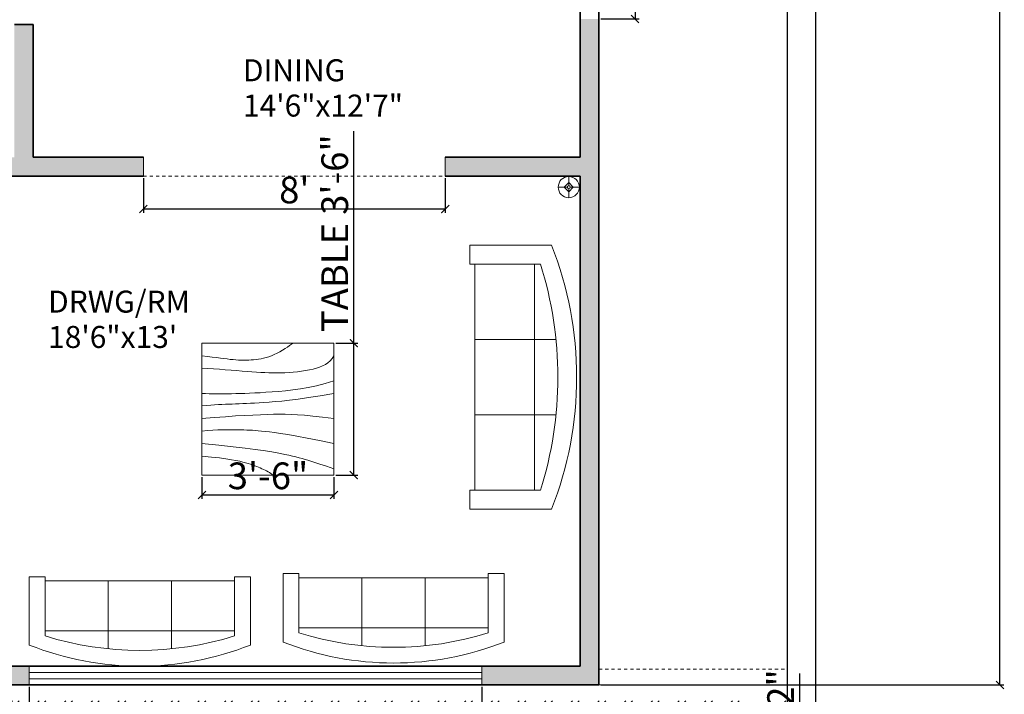
# Model space of a CAD drawing. Units: inches. Extents: x 3799 to 20199, y 1682 to 8087.
# Tile 9 of 30: x 11366 to 11679, y 2322 to 2537. Entities that reach past the tile are written whole.
import ezdxf

# ---------------------------------------------------------------- set-up
doc = ezdxf.new("R2010")
doc.units = ezdxf.units.IN
doc.linetypes.add('JIS_02_1.0', pattern=[2, 1, -1])
for name, color, linetype, lineweight in [('A-ANNO-DIMS', 2, 'Continuous', 18), ('A-AREA-IDEN', 7, 'Continuous', 18), ('A-DOOR', 3, 'Continuous', 18), ('A-FURN', 8, 'Continuous', 18), ('A-GLAZ', 152, 'Continuous', 18), ('A-SITE-OVHD', 8, 'JIS_02_1.0', 18), ('A-WALL', 7, 'Continuous', 35), ('A-WALL-OVHD', 7, 'JIS_02_1.0', 18), ('A-WALL-PATT', 252, 'Continuous', 13), ('C-PROP', 7, 'Continuous', 25), ('L-PLNT-PATT', 94, 'Continuous', 13)]:
    doc.layers.add(name, color=color, linetype=linetype, lineweight=lineweight)
doc.styles.get("Standard").update_dxf_attribs({"font": 'arial.ttf'})
doc.dimstyles.new('ISO-25', dxfattribs={"dimtxt": 8.5, "dimasz": 2.5, "dimexe": 1.25, "dimexo": 0.625, "dimtad": 1, "dimdec": 0, "dimlunit": 3, "dimtxsty": 'Standard', "dimblk": 'ARCHTICK', "dimcen": 2.5, "dimadec": 0, "dimazin": 0, "dimtfac": 1, "dimtdec": 0, "dimtmove": 0, "dimatfit": 3, "dimfxl": 1, "dimarcsym": 0})

# ---------------------------------------------------------------- blocks, each defined once
blk = doc.blocks.new('Sofa - Roundback 7 ft.')
for p, q in [((-12.00002, -32.4421), (-12.00003, -6.5971)), ((11.99997, -32.4421), (11.99998, -6.5971)), ((-36.000027, -34), (-36.000027, -11.4696)), ((35.99998, -34), (35.99998, -11.4696)), ((-35.999844, -13.3819), (35.9998, -13.3819)), ((-36.000027, -32.4421), (35.99998, -32.4421))]:
    blk.add_line(p, q)
for points in [[(-36.000027, -34), (-42.000027, -34), (-42.000027, -8)], [(41.99998, -8), (41.99998, -34), (35.99998, -34)]]:
    blk.add_lwpolyline(points)
for centre, radius, start, end in [((0, -114.25), 114.25, 68.43141, 111.5686), ((-0.00001, -127.1968), 121.1968, 72.72033, 107.2797)]:
    blk.add_arc(centre, radius, start, end)
blk = doc.blocks.new('Table - Square Woodgrain 42 x 42 in.')
blk.add_line((0, -42), (42, -42))
for points in [[(0, -4), (1.704, -4.2172), (3.2358, -4.4188), (4.615, -4.604), (5.8615, -4.7721), (6.9951, -4.9224), (8.0357, -5.0541), (9.0031, -5.1667), (9.9171, -5.2594), (10.7951, -5.3316), (11.6445, -5.3836), (12.4702, -5.4157), (13.277, -5.4283), (14.0698, -5.4217), (14.8535, -5.3964), (15.6331, -5.3526), (16.4133, -5.2908), (17.1986, -5.2103), (17.9913, -5.1062), (18.793, -4.9727), (19.6056, -4.8038), (20.4307, -4.5937), (21.2701, -4.3365), (22.1256, -4.0262), (22.9989, -3.6571), (23.888, -3.2272), (24.7756, -2.7516), (25.6408, -2.2491), (26.4624, -1.7387), (27.2195, -1.2395), (27.891, -0.7703), (28.456, -0.3501), (28.8934, 0.002)], [(0, -42), (0, 0), (42, 0), (42, -42)], [(0, -8), (1.8203, -8.1001), (3.6741, -8.2149), (5.5411, -8.3408), (7.4011, -8.4741), (9.2339, -8.6112), (11.0193, -8.7484), (12.7371, -8.8821), (14.3671, -9.0086), (15.8954, -9.1246), (17.3337, -9.2278), (18.6997, -9.3159), (20.0116, -9.387), (21.2871, -9.4389), (22.5442, -9.4696), (23.8008, -9.477), (25.0749, -9.459), (26.3791, -9.4137), (27.7049, -9.3403), (29.0383, -9.2382), (30.3655, -9.1068), (31.6728, -8.9455), (32.9461, -8.7535), (34.1717, -8.5304), (35.3358, -8.2756), (36.4268, -7.9863), (37.443, -7.6521), (38.3849, -7.2603), (39.253, -6.7986), (40.048, -6.2542), (40.7705, -5.6147), (41.421, -4.8674), (42, -4)], [(42, -12), (39.1784, -12.8621), (36.4519, -13.5654), (33.8246, -14.1294), (31.3004, -14.5731), (28.8832, -14.9161), (26.577, -15.1775), (24.3858, -15.3768), (22.3136, -15.5332), (20.3622, -15.6632), (18.5254, -15.7718), (16.7947, -15.8612), (15.1618, -15.9338), (13.6183, -15.9916), (12.1558, -16.0369), (10.7659, -16.0718), (9.4403, -16.0987), (8.1703, -16.1191), (6.9461, -16.1325), (5.7577, -16.1377), (4.595, -16.1335), (3.4479, -16.1188), (2.3064, -16.0924), (1.1604, -16.0532), (0, -16)], [(42, -16), (37.6529, -16.7365), (33.8802, -17.329), (30.6179, -17.7961), (27.8015, -18.1561), (25.3668, -18.4275), (23.2497, -18.6288), (21.3859, -18.7785), (19.7111, -18.8949), (18.1693, -18.9939), (16.7375, -19.0795), (15.401, -19.1534), (14.1449, -19.217), (12.9544, -19.2717), (11.8148, -19.3191), (10.7113, -19.3606), (9.6291, -19.3976), (8.5534, -19.4323), (7.47, -19.4689), (6.3643, -19.5122), (5.222, -19.5672), (4.0288, -19.6386), (2.7703, -19.7313), (1.4321, -19.8501), (0, -20)], [(0, -24), (3.9243, -23.6805), (7.4766, -23.4138), (10.6891, -23.1954), (13.5943, -23.0205), (16.2247, -22.8847), (18.6125, -22.7832), (20.7903, -22.7116), (22.7903, -22.6651), (24.6563, -22.642), (26.4764, -22.6507), (28.35, -22.7024), (30.3766, -22.8084), (32.6555, -22.98), (35.2861, -23.2283), (38.3678, -23.5645), (42, -24)], [(42, -32), (37.392, -31.017), (33.4585, -30.2231), (30.1291, -29.5949), (27.3334, -29.109), (25.0009, -28.742), (23.0612, -28.4707), (21.4439, -28.2716), (20.0786, -28.1215), (18.8998, -28.0002), (17.8609, -27.9014), (16.9206, -27.8219), (16.0371, -27.7588), (15.1691, -27.709), (14.2748, -27.6693), (13.3128, -27.6368), (12.2415, -27.6083), (11.0295, -27.5824), (9.6867, -27.5643), (8.233, -27.5608), (6.6884, -27.5787), (5.0728, -27.6248), (3.4062, -27.7058), (1.7086, -27.8286), (0, -28)], [(0, -32), (5.4026, -32.5358), (9.9494, -33.019), (13.7424, -33.4553), (16.8834, -33.8505), (19.4743, -34.2106), (21.6171, -34.5413), (23.4136, -34.8486), (24.9657, -35.1382), (26.3614, -35.4156), (27.6332, -35.6841), (28.7995, -35.9467), (29.8788, -36.2064), (30.8897, -36.4661), (31.8507, -36.7288), (32.7802, -36.9973), (33.6968, -37.2747), (34.6175, -37.5635), (35.5531, -37.8651), (36.5128, -38.1805), (37.506, -38.5108), (38.5421, -38.8568), (39.6302, -39.2197), (40.7797, -39.6004), (42, -40)], [(0, -36), (3.0098, -36.2857), (5.5354, -36.5643), (7.6368, -36.8359), (9.374, -37.1009), (10.807, -37.3597), (11.9957, -37.6126), (13.0002, -37.8599), (13.8804, -38.102), (14.6874, -38.3393), (15.4365, -38.5729), (16.1338, -38.8041), (16.7858, -39.0341), (17.3987, -39.264), (17.9787, -39.4952), (18.5322, -39.7288), (19.0655, -39.9662), (19.5832, -40.2081), (20.0842, -40.4544), (20.5657, -40.7046), (21.0249, -40.9581), (21.459, -41.2144), (21.8653, -41.4731), (22.2409, -41.7335), (22.5831, -41.9951)]]:
    blk.add_lwpolyline(points)
blk = doc.blocks.new('_ArchTick')
at = {"color": 0, "linetype": 'ByBlock', "const_width": 0.15}
blk.add_lwpolyline([(-0.5, -0.5), (0.5, 0.5)], dxfattribs=at)
blk = doc.blocks.new('*D58')
at = {"layer": 'A-ANNO-DIMS', "color": 0, "lineweight": -2, "transparency": 16777216}
for p, q in [((11404.92, 2486.45), (11404.92, 2475.33)), ((11500.92, 2486.45), (11500.92, 2475.33)), ((11500.92, 2476.58), (11404.92, 2476.58))]:
    blk.add_line(p, q, dxfattribs=at)
at = {"layer": 'Defpoints', "color": 0, "transparency": 16777216}
for p in [(11404.92, 2487.07), (11500.92, 2487.07), (11404.92, 2476.58)]:
    blk.add_point(p, dxfattribs=at)
at = {"layer": 'A-ANNO-DIMS', "color": 0, "lineweight": -2, "transparency": 16777216, "xscale": 2.5, "yscale": 2.5, "zscale": 2.5, "rotation": 180}
blk.add_blockref('_ArchTick', (11404.92, 2476.58), dxfattribs=at)
at = {"layer": 'A-ANNO-DIMS', "color": 0, "lineweight": -2, "transparency": 16777216, "xscale": 2.5, "yscale": 2.5, "zscale": 2.5}
blk.add_blockref('_ArchTick', (11500.92, 2476.58), dxfattribs=at)
at = {"layer": 'A-ANNO-DIMS', "color": 0, "transparency": 16777216, "insert": (11452.92, 2481.54), "char_height": 8.5, "attachment_point": 5}
blk.add_mtext("8'", dxfattribs=at)
blk = doc.blocks.new('*D70')
at = {"layer": 'A-ANNO-DIMS', "color": 0, "lineweight": -2, "transparency": 16777216}
for p, q in [((11550.48, 2621.07), (11562.6, 2621.07)), ((11561.35, 2621.07), (11561.35, 2537.07)), ((11550.48, 2537.07), (11562.6, 2537.07))]:
    blk.add_line(p, q, dxfattribs=at)
at = {"layer": 'Defpoints', "color": 0, "transparency": 16777216}
for p in [(11549.85, 2621.07), (11549.85, 2537.07), (11561.35, 2537.07)]:
    blk.add_point(p, dxfattribs=at)
at = {"layer": 'A-ANNO-DIMS', "color": 0, "lineweight": -2, "transparency": 16777216, "xscale": 2.5, "yscale": 2.5, "zscale": 2.5}
for p, rotation in [((11561.35, 2621.07), 90), ((11561.35, 2537.07), 270)]:
    blk.add_blockref('_ArchTick', p, dxfattribs=dict(at, rotation=rotation))
at = {"layer": 'A-ANNO-DIMS', "color": 0, "transparency": 16777216, "insert": (11556.48, 2579.07), "char_height": 8.5, "attachment_point": 5, "rotation": 90}
blk.add_mtext("7'", dxfattribs=at)
blk = doc.blocks.new('*D71')
at = {"layer": 'A-ANNO-DIMS', "color": 0, "lineweight": -2, "transparency": 16777216}
for p, q in [((11368.59, 2324.45), (11368.59, 2307.25)), ((11512.59, 2324.45), (11512.59, 2307.25)), ((11368.59, 2308.5), (11512.59, 2308.5))]:
    blk.add_line(p, q, dxfattribs=at)
at = {"layer": 'Defpoints', "color": 0, "transparency": 16777216}
for p in [(11368.59, 2325.07), (11512.59, 2325.07), (11512.59, 2308.5)]:
    blk.add_point(p, dxfattribs=at)
at = {"layer": 'A-ANNO-DIMS', "color": 0, "lineweight": -2, "transparency": 16777216, "xscale": 2.5, "yscale": 2.5, "zscale": 2.5, "rotation": 180}
blk.add_blockref('_ArchTick', (11368.59, 2308.5), dxfattribs=at)
at = {"layer": 'A-ANNO-DIMS', "color": 0, "lineweight": -2, "transparency": 16777216, "xscale": 2.5, "yscale": 2.5, "zscale": 2.5}
blk.add_blockref('_ArchTick', (11512.59, 2308.5), dxfattribs=at)
at = {"layer": 'A-ANNO-DIMS', "color": 0, "transparency": 16777216, "insert": (11440.59, 2313.39), "char_height": 8.5, "attachment_point": 5}
blk.add_mtext("12'", dxfattribs=at)
blk = doc.blocks.new('Lamp - Table')
for p, q in [((0, 7), (0, 1)), ((-1, 0), (-7, 0)), ((0, 3), (-3, 0)), ((-3, 0), (0, -3)), ((3, 0), (0, 3)), ((0, -3), (3, 0)), ((1, 0), (7, 0)), ((0, -1), (0, -7))]:
    blk.add_line(p, q)
for radius in [7, 1]:
    blk.add_circle((0, 0), radius)
blk = doc.blocks.new('WIN-144IN-6IN-FRAME')
for p, q in [((0, 6), (0, 0)), ((144, 4), (0, 4)), ((144, 6), (144, 0)), ((144, 2), (0, 2))]:
    blk.add_line(p, q)
blk = doc.blocks.new('*D346')
at = {"layer": 'A-ANNO-DIMS', "color": 0, "lineweight": -2, "transparency": 16777216}
for p, q in [((11471.84, 2433.89), (11471.84, 2501.37)), ((11466.17, 2433.89), (11473.09, 2433.89)), ((11471.84, 2391.89), (11471.84, 2433.89)), ((11466.17, 2391.89), (11473.09, 2391.89))]:
    blk.add_line(p, q, dxfattribs=at)
at = {"layer": 'Defpoints', "color": 0, "transparency": 16777216}
for p in [(11465.54, 2433.89), (11471.84, 2433.89), (11465.54, 2391.89)]:
    blk.add_point(p, dxfattribs=at)
at = {"layer": 'A-ANNO-DIMS', "color": 0, "lineweight": -2, "transparency": 16777216, "xscale": 2.5, "yscale": 2.5, "zscale": 2.5}
for p, rotation in [((11471.84, 2433.89), 90), ((11471.84, 2391.89), 270)]:
    blk.add_blockref('_ArchTick', p, dxfattribs=dict(at, rotation=rotation))
at = {"layer": 'A-ANNO-DIMS', "color": 0, "transparency": 16777216, "insert": (11466.87, 2468.88), "char_height": 8.5, "attachment_point": 5, "rotation": 90}
blk.add_mtext('TABLE 3\'-6"', dxfattribs=at)
blk = doc.blocks.new('*D347')
at = {"layer": 'A-ANNO-DIMS', "color": 0, "lineweight": -2, "transparency": 16777216}
for p, q in [((11423.54, 2391.26), (11423.54, 2384.34)), ((11465.54, 2391.26), (11465.54, 2384.34)), ((11423.54, 2385.59), (11465.54, 2385.59))]:
    blk.add_line(p, q, dxfattribs=at)
at = {"layer": 'Defpoints', "color": 0, "transparency": 16777216}
for p in [(11423.54, 2391.89), (11465.54, 2391.89), (11465.54, 2385.59)]:
    blk.add_point(p, dxfattribs=at)
at = {"layer": 'A-ANNO-DIMS', "color": 0, "lineweight": -2, "transparency": 16777216, "xscale": 2.5, "yscale": 2.5, "zscale": 2.5, "rotation": 180}
blk.add_blockref('_ArchTick', (11423.54, 2385.59), dxfattribs=at)
at = {"layer": 'A-ANNO-DIMS', "color": 0, "lineweight": -2, "transparency": 16777216, "xscale": 2.5, "yscale": 2.5, "zscale": 2.5}
blk.add_blockref('_ArchTick', (11465.54, 2385.59), dxfattribs=at)
at = {"layer": 'A-ANNO-DIMS', "color": 0, "transparency": 16777216, "insert": (11444.54, 2390.55), "char_height": 8.5, "attachment_point": 5}
blk.add_mtext('3\'-6"', dxfattribs=at)
blk = doc.blocks.new('*D349')
at = {"layer": 'A-ANNO-DIMS', "color": 0, "lineweight": -2, "transparency": 16777216}
for p, q in [((11613.78, 2276.8), (11613.78, 2328.76)), ((11610.46, 2276.8), (11615.03, 2276.8)), ((11613.78, 2253.33), (11613.78, 2276.8)), ((11610.46, 2253.33), (11615.03, 2253.33))]:
    blk.add_line(p, q, dxfattribs=at)
at = {"layer": 'Defpoints', "color": 0, "transparency": 16777216}
for p in [(11609.84, 2276.8), (11613.78, 2276.8), (11609.84, 2253.33)]:
    blk.add_point(p, dxfattribs=at)
at = {"layer": 'A-ANNO-DIMS', "color": 0, "lineweight": -2, "transparency": 16777216, "xscale": 2.5, "yscale": 2.5, "zscale": 2.5}
for p, rotation in [((11613.78, 2276.8), 90), ((11613.78, 2253.33), 270)]:
    blk.add_blockref('_ArchTick', p, dxfattribs=dict(at, rotation=rotation))
at = {"layer": 'A-ANNO-DIMS', "color": 0, "transparency": 16777216, "insert": (11608.76, 2304.03), "char_height": 8.5, "attachment_point": 5, "rotation": 90}
blk.add_mtext('1\'-11 1/2"', dxfattribs=at)
blk = doc.blocks.new('*D374')
at = {"layer": 'A-ANNO-DIMS', "color": 0, "lineweight": -2, "transparency": 16777216}
for p, q in [((11550.48, 3135.07), (11678.7, 3135.07)), ((11677.45, 2325.07), (11677.45, 3135.07)), ((11550.48, 2325.07), (11678.7, 2325.07))]:
    blk.add_line(p, q, dxfattribs=at)
at = {"layer": 'Defpoints', "color": 0, "transparency": 16777216}
for p in [(11549.85, 3135.07), (11677.45, 3135.07), (11549.85, 2325.07)]:
    blk.add_point(p, dxfattribs=at)
at = {"layer": 'A-ANNO-DIMS', "color": 0, "lineweight": -2, "transparency": 16777216, "xscale": 2.5, "yscale": 2.5, "zscale": 2.5}
for p, rotation in [((11677.45, 3135.07), 90), ((11677.45, 2325.07), 270)]:
    blk.add_blockref('_ArchTick', p, dxfattribs=dict(at, rotation=rotation))
at = {"layer": 'A-ANNO-DIMS', "color": 0, "transparency": 16777216, "insert": (11672.49, 2730.07), "char_height": 8.5, "attachment_point": 5, "rotation": 90}
blk.add_mtext('67\'-6"', dxfattribs=at)

msp = doc.modelspace()

# ---------------------------------------------------------------- hatches: boundary and pattern name
at = {"layer": 'A-WALL-PATT'}
h = msp.add_hatch(color=256, dxfattribs=at)
h.dxf.hatch_style = 1
h.paths.add_polyline_path([(11549.85, 2537.07), (11543.85, 2537.07), (11543.85, 2493.07), (11500.92, 2493.07), (11500.92, 2487.07), (11543.85, 2487.07), (11543.85, 2331.07), (11512.59, 2331.07), (11512.59, 2325.07), (11549.85, 2325.07)])
h.paths.add_polyline_path([(11404.92, 2493.07), (11369.85, 2493.07), (11369.85, 2535.29), (11363.85, 2535.29), (11363.85, 2493.07), (11359.67, 2493.07), (11359.67, 2487.07), (11404.92, 2487.07)])
h.paths.add_polyline_path([(11347.67, 2493.07), (11315.85, 2493.07), (11315.85, 2481.32), (11321.85, 2481.32), (11321.85, 2487.07), (11347.67, 2487.07)])
h.paths.add_polyline_path([(11246.96, 2394.07), (11231.85, 2394.07), (11231.85, 2493.07), (11126.81, 2493.07), (11126.81, 2487.07), (11225.85, 2487.07), (11225.85, 2325.07), (11315.85, 2325.07), (11315.85, 2331.07), (11231.85, 2331.07), (11231.85, 2388.07), (11246.96, 2388.07)])
h.paths.add_polyline_path([(11368.59, 2331.07), (11321.85, 2331.07), (11321.85, 2421.32), (11319.79, 2421.32), (11315.85, 2421.32), (11315.85, 2394.07), (11306.96, 2394.07), (11306.96, 2392.01), (11306.96, 2388.07), (11315.85, 2388.07), (11315.85, 2325.07), (11368.59, 2325.07)])
h.paths.add_polyline_path([(11211.5, 2599.62), (11175.25, 2599.62), (11175.25, 2594.62), (11206.5, 2594.62), (11206.5, 2541.62), (11137.5, 2541.62), (11137.5, 2594.62), (11145.25, 2594.62), (11145.25, 2599.62), (11132.5, 2599.62), (11132.5, 2536.62), (11211.5, 2536.62)], flags=17)
h.paths.add_polyline_path([(11278.96, 2650.07), (11117.85, 2650.07), (11117.85, 2668.07), (11111.85, 2668.07), (11111.85, 2650.07), (11087.85, 2650.07), (11087.85, 2526.57), (11093.85, 2526.57), (11093.85, 2644.07), (11278.96, 2644.07)])
h.paths.add_polyline_path([(11096.81, 2491.01), (11096.81, 2493.07), (11093.85, 2493.07), (11093.85, 2496.57), (11087.85, 2496.57), (11087.85, 2487.07), (11096.81, 2487.07)])
h.paths.add_polyline_path([(11445.85, 3087.71), (11439.85, 3087.71), (11439.85, 2949.07), (11343.85, 2949.07), (11343.85, 2929.61), (11315.6, 2929.61), (11315.6, 2923.61), (11343.85, 2923.61), (11343.85, 2840.12), (11349.85, 2840.12), (11349.85, 2943.07), (11507.11, 2943.07), (11507.11, 2949.07), (11445.85, 2949.07), (11445.85, 3015.07), (11543.85, 3015.07), (11543.85, 2992.92), (11549.85, 2992.92), (11549.85, 3108.28), (11543.85, 3108.28), (11543.85, 3021.07), (11515.89, 3021.07), (11515.89, 3049.36), (11511.89, 3049.36), (11511.89, 3021.07), (11445.85, 3021.07)])
h.paths.add_polyline_path([(11549.85, 3135.07), (11408.12, 3135.07), (11408.12, 3129.07), (11439.85, 3129.07), (11439.85, 3117.71), (11443.79, 3117.71), (11445.85, 3117.71), (11445.85, 3129.07), (11504.47, 3129.07), (11504.47, 3099.65), (11508.47, 3099.65), (11508.47, 3129.07), (11543.85, 3129.07), (11543.85, 3126.28), (11549.85, 3126.28)])
h.paths.add_polyline_path([(11324.12, 3135.07), (11087.85, 3135.07), (11087.85, 3083.46), (11093.85, 3083.46), (11093.85, 3129.07), (11265.85, 3129.07), (11265.85, 3050.07), (11240.75, 3050.07), (11240.75, 3044.07), (11265.85, 3044.07), (11265.85, 2895.64), (11271.85, 2895.64), (11271.85, 2923.61), (11279.6, 2923.61), (11279.6, 2929.61), (11271.85, 2929.61), (11271.85, 3129.07), (11324.12, 3129.07)])
h.paths.add_polyline_path([(11210.75, 3050.07), (11133.85, 3050.07), (11133.85, 3088.63), (11129.85, 3088.54), (11129.85, 3050.07), (11093.85, 3050.07), (11093.85, 3059.46), (11087.85, 3059.46), (11087.85, 3030.25), (11093.85, 3030.25), (11093.85, 3044.07), (11210.75, 3044.07)], flags=17)
h.paths.add_polyline_path([(11093.85, 2982.25), (11087.85, 2982.25), (11087.85, 2913.95), (11093.85, 2913.95)], flags=17)
h.paths.add_polyline_path([(11271.85, 2859.64), (11265.85, 2859.64), (11265.85, 2854.07), (11093.85, 2854.07), (11093.85, 2865.95), (11087.85, 2865.95), (11087.85, 2848.07), (11111.85, 2848.07), (11111.85, 2812.07), (11117.85, 2812.07), (11117.85, 2848.07), (11271.85, 2848.07)])
h.paths.add_polyline_path([(11549.85, 2847.23), (11543.85, 2847.23), (11543.85, 2799.07), (11349.85, 2799.07), (11349.85, 2804.12), (11343.85, 2804.12), (11343.85, 2753.07), (11349.85, 2753.07), (11349.85, 2793.07), (11543.85, 2793.07), (11543.85, 2752.31), (11549.85, 2752.31)])
h.paths.add_polyline_path([(11549.85, 2692.31), (11543.85, 2692.31), (11543.85, 2650.07), (11343.85, 2650.07), (11338.96, 2650.07), (11338.96, 2644.07), (11349.85, 2644.07), (11363.85, 2644.07), (11363.85, 2608.29), (11369.85, 2608.29), (11369.85, 2644.07), (11543.85, 2644.07), (11543.85, 2621.07), (11549.85, 2621.07)])
at = {"layer": 'L-PLNT-PATT'}
h = msp.add_hatch(dxfattribs=at)
h.set_pattern_fill('GOST_GLASS', color=256)
h.paths.add_polyline_path([(11609.85, 2325.07), (11549.85, 2325.07), (11315.85, 2325.07), (11315.85, 2300.82), (11302.02, 2300.82), (11302.02, 2133.07), (11609.85, 2133.07)])
h.paths.add_polyline_path([(11496.55, 2144.31), (11496.62, 2144.39), (11496.58, 2144.52)], flags=16)
h.paths.add_polyline_path([(11491.91, 2145.12), (11493.01, 2143.36), (11494.28, 2143.99), (11494.28, 2144.01), (11494.36, 2143.39), (11494.73, 2142.84), (11494.91, 2142.94), (11495.46, 2143.67), (11495.33, 2142.52), (11496.19, 2140.15), (11495.75, 2139.78), (11494.7, 2136.83), (11492.98, 2136.07), (11493.22, 2135.99), (11492.8, 2135.99), (11491.54, 2136.62), (11490.91, 2137.68), (11490.07, 2138.1), (11489.64, 2139.15), (11489.22, 2141.04), (11489.22, 2142.73), (11489.64, 2143.71), (11490.07, 2143.57), (11491.02, 2144.77), (11491.12, 2144.24), (11491.46, 2143.95), (11491.73, 2144.28)], flags=16)
h.paths.add_polyline_path([(11491.31, 2142.42), (11493.01, 2140.83), (11492.8, 2138.94), (11491.96, 2137.47), (11490.91, 2141.04), (11491.77, 2141.99), (11490.77, 2142.92), (11491.35, 2143.4)], flags=0)
h.paths.add_polyline_path([(11455.55, 2140.87), (11453.52, 2140.87), (11451.69, 2140.04), (11455.54, 2140.52, 0.011687)], flags=16)
h.paths.add_polyline_path([(11451.82, 2137.03), (11451.82, 2136.94), (11451.92, 2136.93)], flags=16)
h.paths.add_polyline_path([(11447.97, 2140.87), (11447.97, 2135.62), (11447.21, 2136.28), (11446.7, 2139.6), (11446.1, 2139), (11446.11, 2136.84), (11446.26, 2136.47), (11446.11, 2136.28), (11446.12, 2134.9), (11445.36, 2134.39), (11445.25, 2135.18), (11446.11, 2136.28), (11446.1, 2138.85), (11445.88, 2138.78), (11443.88, 2136.78), (11442.77, 2136.56), (11443.44, 2138.06), (11441.62, 2137.52), (11442.08, 2138.6), (11442.26, 2138.61), (11442, 2138.42), (11441.62, 2137.52), (11445.88, 2138.78), (11447.97, 2140.87), (11447.97, 2143.39), (11445.18, 2146.18), (11445.72, 2147.71), (11447.97, 2146.55), (11447.97, 2148.2), (11448.27, 2147.82), (11448.02, 2146.98), (11450.07, 2142.97)], flags=16)
h.paths.add_polyline_path([(11551.41, 2140.65, -1), (11536.26, 2140.65, -1)])
h.paths.add_polyline_path([(11547.68, 2136.8), (11547.69, 2136.71), (11547.78, 2136.7)], flags=16)
h.paths.add_polyline_path([(11541.05, 2145.95), (11541.58, 2147.48), (11542.26, 2147.14), (11542.27, 2144.73)], flags=16)
h.paths.add_polyline_path([(11541.96, 2138.78), (11541.97, 2136.62), (11542.12, 2136.24), (11541.97, 2136.06), (11541.98, 2134.67), (11541.23, 2134.17), (11541.11, 2134.95), (11541.97, 2136.06), (11541.96, 2138.62), (11541.74, 2138.56), (11539.74, 2136.56), (11538.63, 2136.33), (11539.3, 2137.83), (11537.48, 2137.29), (11537.94, 2138.37), (11538.12, 2138.38), (11541.25, 2140.65), (11543.83, 2140.65)], flags=16)
h.paths.add_polyline_path([(11584.29, 2268.01), (11584.1, 2268.75), (11584.25, 2269.39), (11584.02, 2270.08), (11583.56, 2270.33), (11584.06, 2270.63), (11584.18, 2271.22), (11584.1, 2271.81), (11584.48, 2272.21), (11584.83, 2272.85), (11584.45, 2273.49), (11583.87, 2273.79), (11584.72, 2273.79), (11585.41, 2273.89), (11585.79, 2274.33), (11585.79, 2274.73), (11586.3, 2275.17), (11587.03, 2275.22), (11587.76, 2275.66), (11588.26, 2275.62), (11588.72, 2275.91), (11589.22, 2275.66), (11589.53, 2276.8), (11589.69, 2275.91), (11590.23, 2275.81), (11590.92, 2276.11), (11591.46, 2276.26), (11592.73, 2275.22), (11593.19, 2274.92), (11593.58, 2275.12), (11594.35, 2274.87), (11594.31, 2274.38), (11594.43, 2274.03), (11595.08, 2273.34), (11595.47, 2272.9), (11595.54, 2271.76), (11595.89, 2271.47), (11596.85, 2271.47), (11597.55, 2271.52), (11596.78, 2271.22), (11596.08, 2270.87), (11595.93, 2270.43), (11596.04, 2269.79), (11595.85, 2269.58), (11596.25, 2269.39), (11596.63, 2270.81), (11596.82, 2269.7), (11597.5, 2269.57), (11598.36, 2269.94), (11599.04, 2270.13), (11600.63, 2268.83), (11601.21, 2268.46), (11601.77, 2268.75), (11601.65, 2268.95), (11601.29, 2269.14), (11601.82, 2269.14), (11602.25, 2269.2), (11602.49, 2269.48), (11602.49, 2269.72), (11602.81, 2270), (11603.26, 2270.03), (11603.72, 2270.31), (11604.04, 2270.28), (11604.32, 2270.46), (11604.64, 2270.31), (11604.83, 2271.02), (11604.93, 2270.46), (11605.26, 2270.4), (11605.7, 2270.59), (11606.03, 2270.68), (11606.83, 2270.03), (11607.12, 2269.85), (11607.36, 2269.97), (11607.84, 2269.82), (11607.82, 2269.51), (11607.89, 2269.29), (11608.3, 2268.86), (11608.54, 2268.58), (11608.59, 2267.87), (11608.8, 2267.68), (11609.4, 2267.68), (11609.84, 2267.72), (11609.36, 2267.53), (11608.92, 2267.31), (11608.83, 2267.04), (11608.9, 2266.64), (11608.73, 2266.45), (11608.63, 2265.68), (11608.75, 2265.52), (11608.66, 2265.46), (11608.44, 2265.04), (11608.03, 2264.97), (11608.39, 2264.54), (11607.96, 2264.63), (11607.84, 2264.57), (11607.82, 2264.32), (11607.45, 2263.98), (11607.26, 2263.7), (11606.85, 2263.64), (11606.54, 2263.39), (11606.01, 2263.24), (11605.65, 2263.27), (11605.31, 2263.15), (11605.21, 2263.02), (11605.12, 2262.28), (11604.9, 2263.02), (11604.71, 2263.08), (11604.63, 2262.84), (11604.77, 2262.04), (11604.43, 2261.67), (11604.24, 2260.13), (11604.48, 2259.82), (11604.29, 2259.69), (11604, 2259.14), (11603.76, 2258.83), (11603.04, 2258.71), (11603.76, 2257.84), (11602.89, 2258.03), (11602.65, 2257.9), (11602.6, 2257.41), (11601.88, 2256.73), (11601.49, 2256.17), (11600.68, 2256.05), (11600.05, 2255.56), (11598.99, 2255.25), (11598.27, 2255.31), (11597.59, 2255.06), (11597.4, 2254.82), (11597.21, 2253.33), (11596.77, 2254.82), (11595.19, 2255.25), (11594.51, 2255.31), (11593.79, 2255.87), (11593.21, 2256.48), (11592.73, 2256.61), (11592.1, 2256.17), (11591.48, 2255.56), (11591.81, 2256.36), (11591.91, 2257.47), (11591.53, 2257.96), (11590.75, 2258.34), (11590.75, 2258.95), (11590.61, 2259.45), (11590.08, 2259.82), (11589.84, 2260.74), (11590.03, 2261.55), (11589.74, 2262.41), (11589.17, 2262.72), (11589.79, 2263.09), (11589.84, 2263.34), (11589.65, 2264.01), (11588.38, 2264.35), (11587.84, 2264.4), (11587.26, 2264.85), (11586.8, 2265.34), (11586.41, 2265.44), (11585.91, 2265.09), (11585.41, 2264.6), (11585.68, 2265.24), (11585.76, 2266.13), (11585.45, 2266.53), (11584.83, 2266.82), (11584.83, 2267.32), (11584.72, 2267.71)], flags=16)
h.paths.add_polyline_path([(11589.76, 2270.08), (11589.88, 2270.23), (11589.99, 2270.08)], flags=0)
h.paths.add_polyline_path([(11596.92, 2262.41), (11597.06, 2262.6), (11597.21, 2262.41)], flags=0)
h.paths.add_polyline_path([(11607.36, 2210.31), (11607.43, 2210.39), (11607.39, 2210.52)], flags=16)
h.paths.add_polyline_path([(11600.87, 2204.1), (11600.45, 2205.15), (11600.03, 2207.04), (11600.03, 2208.73), (11600.45, 2209.71), (11600.87, 2209.57), (11601.83, 2210.77), (11601.93, 2210.24), (11602.27, 2209.95), (11602.54, 2210.28), (11602.72, 2211.12), (11603.82, 2209.36), (11605.09, 2209.99), (11605.09, 2210), (11605.17, 2209.39), (11605.54, 2208.84), (11605.72, 2208.94), (11606.27, 2209.67), (11606.14, 2208.52), (11607, 2206.15), (11606.56, 2205.78), (11605.51, 2202.83), (11603.79, 2202.07), (11604.03, 2201.99), (11603.61, 2201.99), (11602.35, 2202.62), (11601.72, 2203.68)], flags=16)
h.paths.add_polyline_path([(11601.72, 2207.04), (11602.58, 2207.99), (11601.57, 2208.92), (11602.16, 2209.4), (11602.12, 2208.42), (11603.82, 2206.83), (11603.61, 2204.94), (11602.77, 2203.47)], flags=0)
h.paths.add_polyline_path([(11399.57, 2144.02), (11399.64, 2144.1), (11399.6, 2144.23)], flags=16)
h.paths.add_polyline_path([(11398.77, 2139.49), (11397.71, 2136.54), (11396, 2135.78), (11396.24, 2135.7), (11395.82, 2135.7), (11394.55, 2136.33), (11393.92, 2137.38), (11393.08, 2137.81), (11392.66, 2138.86), (11392.24, 2140.75), (11392.24, 2142.44), (11392.66, 2143.42), (11393.08, 2143.28), (11394.04, 2144.48), (11394.14, 2143.95), (11394.47, 2143.66), (11394.74, 2143.99), (11394.93, 2144.83), (11396.03, 2143.07), (11397.29, 2143.7), (11397.3, 2143.71), (11397.37, 2143.1), (11397.75, 2142.55), (11397.92, 2142.65), (11398.47, 2143.38), (11398.34, 2142.23), (11399.21, 2139.86)], flags=16)
h.paths.add_polyline_path([(11609.04, 2180.55, -1), (11593.89, 2180.55, -1)], flags=16)
h.paths.add_polyline_path([(11605.31, 2176.71), (11605.32, 2176.61), (11605.41, 2176.6)], flags=0)
h.paths.add_polyline_path([(11601.47, 2180.55), (11601.47, 2183.07), (11598.68, 2185.85), (11599.22, 2187.38), (11601.47, 2186.23), (11601.47, 2187.88), (11601.76, 2187.5), (11601.52, 2186.66), (11603.57, 2182.65), (11601.47, 2180.55), (11601.47, 2175.3), (11600.7, 2175.96), (11600.2, 2179.28), (11599.6, 2178.68), (11599.61, 2176.52), (11599.75, 2176.15), (11599.61, 2175.96), (11599.61, 2174.57), (11598.86, 2174.07), (11598.74, 2174.85), (11599.61, 2175.96), (11599.6, 2178.53), (11599.38, 2178.46), (11597.38, 2176.46), (11596.27, 2176.23), (11596.94, 2177.74), (11595.11, 2177.19), (11595.58, 2178.28), (11595.76, 2178.28), (11598.89, 2180.55)], flags=0)
h.paths.add_polyline_path([(11394.33, 2142.12), (11396.03, 2140.54), (11395.82, 2138.65), (11394.98, 2137.17), (11393.92, 2140.75), (11394.78, 2141.7), (11393.78, 2142.63), (11394.36, 2143.11)], flags=0)
h.paths.add_polyline_path([(11604.97, 2266.82), (11605.05, 2266.91), (11605.12, 2266.82)], flags=0)
h.paths.add_polyline_path([(11593.36, 2312.93, -1), (11608.51, 2312.93, -1)], flags=16)
h.paths.add_polyline_path([(11604.78, 2309.09), (11604.79, 2309), (11604.88, 2308.99)], flags=0)
h.paths.add_polyline_path([(11596.4, 2310.12), (11594.58, 2309.58), (11595.04, 2310.66), (11595.22, 2310.66), (11598.35, 2312.93), (11600.93, 2312.93), (11600.93, 2315.45), (11598.15, 2318.23), (11598.68, 2319.77), (11600.93, 2318.61), (11600.93, 2320.26), (11601.23, 2319.88), (11600.99, 2319.04), (11603.03, 2315.03), (11600.93, 2312.93), (11600.93, 2307.68), (11600.17, 2308.34), (11599.66, 2311.66), (11599.06, 2311.06), (11599.07, 2308.9), (11599.22, 2308.53), (11599.07, 2308.34), (11599.08, 2306.96), (11598.33, 2306.45), (11598.21, 2307.24), (11599.07, 2308.34), (11599.06, 2310.91), (11598.84, 2310.84), (11596.84, 2308.84), (11595.73, 2308.62)], flags=0)
h.paths.add_polyline_path([(11605.66, 2145.72), (11605.73, 2145.8), (11605.69, 2145.93)], flags=16)
h.paths.add_polyline_path([(11598.75, 2140.56), (11598.33, 2142.46), (11598.33, 2144.14), (11598.75, 2145.12), (11599.17, 2144.98), (11600.13, 2146.18), (11600.23, 2145.66), (11600.56, 2145.36), (11600.83, 2145.69), (11601.02, 2146.53), (11602.12, 2144.77), (11603.38, 2145.4), (11603.39, 2145.42), (11603.46, 2144.81), (11603.84, 2144.25), (11604.02, 2144.35), (11604.56, 2145.08), (11604.44, 2143.93), (11605.3, 2141.56), (11604.86, 2141.19), (11603.8, 2138.25), (11602.09, 2137.48), (11602.33, 2137.4), (11601.91, 2137.4), (11600.65, 2138.04), (11600.01, 2139.09), (11599.17, 2139.51)], flags=16)
h.paths.add_polyline_path([(11600.01, 2142.46), (11600.87, 2143.4), (11599.87, 2144.33), (11600.45, 2144.81), (11600.42, 2143.83), (11602.12, 2142.25), (11601.91, 2140.35), (11601.07, 2138.88)], flags=0)
h.paths.add_polyline_path([(11363.83, 2141.59, -1), (11348.68, 2141.59, -1)], flags=0)
h.paths.add_polyline_path([(11360.1, 2137.75), (11360.11, 2137.66), (11360.2, 2137.65)], flags=0)
h.paths.add_polyline_path([(11356.26, 2141.59), (11356.26, 2136.34), (11355.49, 2137), (11354.98, 2140.32), (11354.38, 2139.72), (11354.39, 2137.56), (11354.54, 2137.19), (11354.39, 2137), (11354.4, 2135.62), (11353.65, 2135.11), (11353.53, 2135.9), (11354.39, 2137), (11354.38, 2139.57), (11354.17, 2139.5), (11352.16, 2137.5), (11351.05, 2137.28), (11351.73, 2138.78), (11349.9, 2138.24), (11350.36, 2139.32), (11350.54, 2139.33), (11353.68, 2141.59), (11356.26, 2141.59), (11356.26, 2144.11), (11353.47, 2146.9), (11354.01, 2148.43), (11356.26, 2147.27), (11356.26, 2148.92), (11356.55, 2148.54), (11356.31, 2147.7), (11358.35, 2143.69)], flags=0)
h.paths.add_polyline_path([(11313.11, 2243.68), (11313.18, 2243.77), (11313.14, 2243.89)], flags=16)
h.paths.add_polyline_path([(11312.31, 2239.16), (11311.26, 2236.21), (11309.55, 2235.45), (11309.79, 2235.37), (11309.37, 2235.37), (11308.1, 2236), (11307.47, 2237.05), (11306.63, 2237.47), (11306.21, 2238.53), (11305.79, 2240.42), (11305.79, 2242.11), (11306.21, 2243.09), (11306.63, 2242.95), (11307.59, 2244.15), (11307.68, 2243.62), (11308.02, 2243.32), (11308.29, 2243.65), (11308.47, 2244.5), (11309.58, 2242.74), (11310.84, 2243.37), (11310.85, 2243.38), (11310.92, 2242.77), (11311.3, 2242.22), (11311.47, 2242.32), (11312.02, 2243.05), (11311.89, 2241.9), (11312.75, 2239.53)], flags=16)
h.paths.add_polyline_path([(11308.52, 2236.84), (11307.47, 2240.42), (11308.33, 2241.37), (11307.33, 2242.3), (11307.91, 2242.78), (11307.87, 2241.79), (11309.58, 2240.21), (11309.37, 2238.32)], flags=0)
h.paths.add_polyline_path([(11302.02, 2281.94, -1), (11317.17, 2281.94, -1)])
h.paths.add_polyline_path([(11313.44, 2278.1), (11313.44, 2278), (11313.54, 2277.99)], flags=16)
h.paths.add_polyline_path([(11309.59, 2276.69), (11308.83, 2277.35), (11308.32, 2280.67), (11307.72, 2280.07), (11307.73, 2277.91), (11307.88, 2277.54), (11307.73, 2277.35), (11307.74, 2275.96), (11306.98, 2275.46), (11306.87, 2276.24), (11307.73, 2277.35), (11307.72, 2279.92), (11307.5, 2279.85), (11305.5, 2277.85), (11304.39, 2277.63), (11305.06, 2279.13), (11303.24, 2278.58), (11303.7, 2279.67), (11303.88, 2279.67), (11303.62, 2279.49), (11303.24, 2278.58), (11307.5, 2279.85), (11309.59, 2281.94), (11309.59, 2284.46), (11306.8, 2287.24), (11307.34, 2288.77), (11309.59, 2287.62), (11309.59, 2289.27), (11309.89, 2288.89), (11309.64, 2288.05), (11311.69, 2284.04), (11309.59, 2281.94)], flags=16)
h.paths.add_polyline_path([(11317.17, 2181.83, -1), (11302.02, 2181.83, -1)])
h.paths.add_polyline_path([(11313.44, 2177.98), (11313.44, 2177.89), (11313.54, 2177.88)], flags=16)
h.paths.add_polyline_path([(11309.59, 2181.83), (11309.59, 2176.58), (11308.83, 2177.24), (11308.32, 2180.56), (11307.72, 2179.96), (11307.73, 2177.8), (11307.88, 2177.42), (11307.73, 2177.24), (11307.74, 2175.85), (11306.98, 2175.35), (11306.87, 2176.13), (11307.73, 2177.24), (11307.72, 2179.8), (11307.5, 2179.74), (11305.5, 2177.74), (11304.39, 2177.51), (11305.06, 2179.01), (11303.24, 2178.47), (11303.7, 2179.55), (11303.88, 2179.56), (11303.62, 2179.38), (11303.24, 2178.47), (11307.5, 2179.74), (11309.59, 2181.83), (11309.59, 2184.35), (11306.8, 2187.13), (11307.34, 2188.66), (11309.59, 2187.51), (11309.59, 2189.16), (11309.89, 2188.78), (11309.64, 2187.94), (11311.69, 2183.93)], flags=16)
h.paths.add_polyline_path([(11318.27, 2141.81), (11318.34, 2141.89), (11318.3, 2142.02)], flags=16)
h.paths.add_polyline_path([(11317.47, 2137.28), (11316.41, 2134.34), (11314.7, 2133.57), (11314.94, 2133.49), (11314.52, 2133.49), (11313.26, 2134.12), (11312.62, 2135.18), (11311.78, 2135.6), (11311.36, 2136.65), (11310.94, 2138.55), (11310.94, 2140.23), (11311.36, 2141.21), (11311.78, 2141.07), (11312.74, 2142.27), (11312.84, 2141.75), (11313.17, 2141.45), (11313.44, 2141.78), (11313.63, 2142.62), (11314.73, 2140.86), (11315.99, 2141.49), (11316, 2141.51), (11316.07, 2140.9), (11316.45, 2140.34), (11316.62, 2140.44), (11317.17, 2141.17), (11317.05, 2140.02), (11317.91, 2137.65)], flags=16)
h.paths.add_polyline_path([(11314.73, 2138.34), (11314.52, 2136.44), (11313.68, 2134.97), (11312.62, 2138.55), (11313.48, 2139.49), (11312.48, 2140.42), (11313.06, 2140.9), (11313.03, 2139.92)], flags=0)
h.paths.add_polyline_path([(11454.71, 2144.33), (11450.92, 2143.82), (11447.97, 2140.87), (11455.55, 2140.87, 0.119183)], flags=16)
h.paths.add_polyline_path([(11450.07, 2142.97), (11448.02, 2146.98), (11447.97, 2147.09), (11447.97, 2146.55), (11447.97, 2140.87)], flags=0)
h.paths.add_polyline_path([(11447.97, 2143.39), (11445.18, 2146.18), (11445.72, 2147.71), (11445.88, 2148.15, 0.334379), (11440.4, 2140.87), (11447.97, 2140.87)], flags=0)
h.paths.add_polyline_path([(11447.97, 2143.39), (11447.97, 2146.55), (11447.97, 2148.45, 0.414214), (11440.4, 2140.87), (11447.97, 2140.87)], flags=16)
h.paths.add_polyline_path([(11447.97, 2138.46), (11447.97, 2135.62), (11447.97, 2133.3, 0.158969), (11452.44, 2134.75), (11450.84, 2136.28), (11451.1, 2135.2), (11450.97, 2134.44)], flags=16)
h.paths.add_polyline_path([(11348.68, 2141.59, 1), (11363.83, 2141.59, 1)], flags=16)
h.paths.add_polyline_path([(11360.1, 2137.75), (11360.28, 2135.9), (11359.13, 2137), (11358.61, 2139.24)], flags=0)
h.paths.add_polyline_path([(11362.99, 2145.05), (11359.2, 2144.54), (11356.26, 2141.59), (11361.81, 2141.59), (11363.78, 2142.49, 0.08904)], flags=0)

# ---------------------------------------------------------------- linework, layer by layer
at = {"layer": 'A-DOOR'}
for p, q in [((11404.92, 2493.07), (11404.92, 2487.07)), ((11500.92, 2493.07), (11500.92, 2487.07))]:
    msp.add_line(p, q, dxfattribs=at)
at = {"layer": 'A-SITE-OVHD'}
for p, q in [((11549.85, 2330.07), (11609.85, 2330.07)), ((11549.85, 2325.07), (11609.85, 2325.07))]:
    msp.add_line(p, q, dxfattribs=at)
at = {"layer": 'A-WALL'}
for p, q in [((11549.85, 2325.07), (11549.85, 3135.07)), ((11543.85, 2493.07), (11543.85, 2644.07)), ((11363.85, 2535.29), (11369.85, 2535.29)), ((11369.85, 2493.07), (11369.85, 2535.29)), ((11369.85, 2493.07), (11404.92, 2493.07)), ((11500.92, 2493.07), (11543.85, 2493.07)), ((11404.92, 2487.07), (11321.85, 2487.07)), ((11543.85, 2487.07), (11500.92, 2487.07)), ((11543.85, 2331.07), (11543.85, 2487.07)), ((11543.85, 2331.07), (11321.85, 2331.07)), ((11549.85, 2325.07), (11315.85, 2325.07))]:
    msp.add_line(p, q, dxfattribs=at)
at = {"layer": 'A-WALL-OVHD'}
msp.add_line((11404.92, 2487.07), (11500.92, 2487.07), dxfattribs=at)
at = {"layer": 'C-PROP'}
for p, q in [((11618.85, 2124.07), (11618.85, 3204.07)), ((11609.85, 2133.07), (11609.85, 3195.07))]:
    msp.add_line(p, q, dxfattribs=at)

# ---------------------------------------------------------------- block references
at = {"layer": 'A-FURN', "xscale": 0.4812244018485111, "yscale": 0.4812244018485111, "zscale": 0.4812244018485111}
msp.add_blockref('Lamp - Table', (11540.25, 2483.54), dxfattribs=at)
at = {"layer": 'A-FURN', "rotation": 270}
msp.add_blockref('Sofa - Roundback 7 ft.', (11542.75, 2423.04), dxfattribs=at)
at = {"layer": 'A-FURN'}
msp.add_blockref('Table - Square Woodgrain 42 x 42 in.', (11423.54, 2433.89), dxfattribs=at)
at = {"layer": 'A-FURN', "xscale": 0.8372446880612686, "yscale": 0.8372446880612686, "zscale": 0.8372446880612686, "rotation": 180}
for p in [(11403.76, 2331.07), (11484.5, 2332.05)]:
    msp.add_blockref('Sofa - Roundback 7 ft.', p, dxfattribs=at)
at = {"layer": 'A-GLAZ'}
msp.add_blockref('WIN-144IN-6IN-FRAME', (11368.59, 2325.07), dxfattribs=at)

# ---------------------------------------------------------------- texts
at = {"layer": 'A-AREA-IDEN'}
for s, p in [('DINING', (11436.57, 2517.24)), ('14\'6"x12\'7"', (11436.57, 2506)), ('DRWG/RM', (11374.56, 2443.6)), ('18\'6"x13\'', (11374.56, 2432.35))]:
    msp.add_text(s, height=7, rotation=0.0019, dxfattribs=at).set_placement(p)

# ---------------------------------------------------------------- dimensions: what is measured, and where the dimension line sits
at = {"layer": 'A-ANNO-DIMS'}
for base, p1, p2, override, picture, middle in [((11677.45, 3135.07), (11549.85, 2325.07), (11549.85, 3135.07), {"dimdec": 1, "dimlfac": 1, "dimrnd": 0, "dimzin": 1, "dimdsep": 46, "dimlunit": 4, "dimfrac": 2}, '*D374', (11672.49, 2730.07)), ((11561.35, 2537.07), (11549.85, 2621.07), (11549.85, 2537.07), {"dimclrd": 0, "dimclre": 0, "dimclrt": 0}, '*D70', (11556.48, 2579.07)), ((11613.78, 2276.8), (11609.84, 2253.33), (11609.84, 2276.8), {"dimdec": 1, "dimlfac": 1, "dimrnd": 0, "dimzin": 1, "dimdsep": 46, "dimlunit": 4, "dimfrac": 2}, '*D349', (11608.76, 2304.03))]:
    dim = msp.add_linear_dim(base=base, p1=p1, p2=p2, angle=90, dimstyle='ISO-25', override=override, dxfattribs=at)
    dim.commit()
    dim.dimension.update_dxf_attribs({"geometry": picture, "text_midpoint": middle})
dim = msp.add_linear_dim(base=(11471.84, 2433.89), p1=(11465.54, 2391.89), p2=(11465.54, 2433.89), angle=90, text='TABLE <>', dimstyle='ISO-25', override={"dimdec": 1, "dimlfac": 1, "dimrnd": 0, "dimzin": 1, "dimdsep": 46, "dimlunit": 4, "dimfrac": 2}, dxfattribs=at)
dim.commit()
dim.dimension.update_dxf_attribs({"geometry": '*D346', "text_midpoint": (11466.87, 2468.88)})
for base, p1, p2, override, picture, middle in [((11404.92, 2476.58), (11500.92, 2487.07), (11404.92, 2487.07), {"dimclrd": 0, "dimclre": 0, "dimclrt": 0}, '*D58', (11452.92, 2481.54)), ((11465.54, 2385.59), (11423.54, 2391.89), (11465.54, 2391.89), {"dimdec": 1, "dimlfac": 1, "dimrnd": 0, "dimzin": 1, "dimdsep": 46, "dimlunit": 4, "dimfrac": 2}, '*D347', (11444.54, 2390.55)), ((11512.59, 2308.5), (11368.59, 2325.07), (11512.59, 2325.07), {"dimclrd": 0, "dimclre": 0, "dimclrt": 0}, '*D71', (11440.59, 2313.39))]:
    dim = msp.add_linear_dim(base=base, p1=p1, p2=p2, dimstyle='ISO-25', override=override, dxfattribs=at)
    dim.commit()
    dim.dimension.update_dxf_attribs({"geometry": picture, "text_midpoint": middle})

doc.saveas('drawing.dxf')
